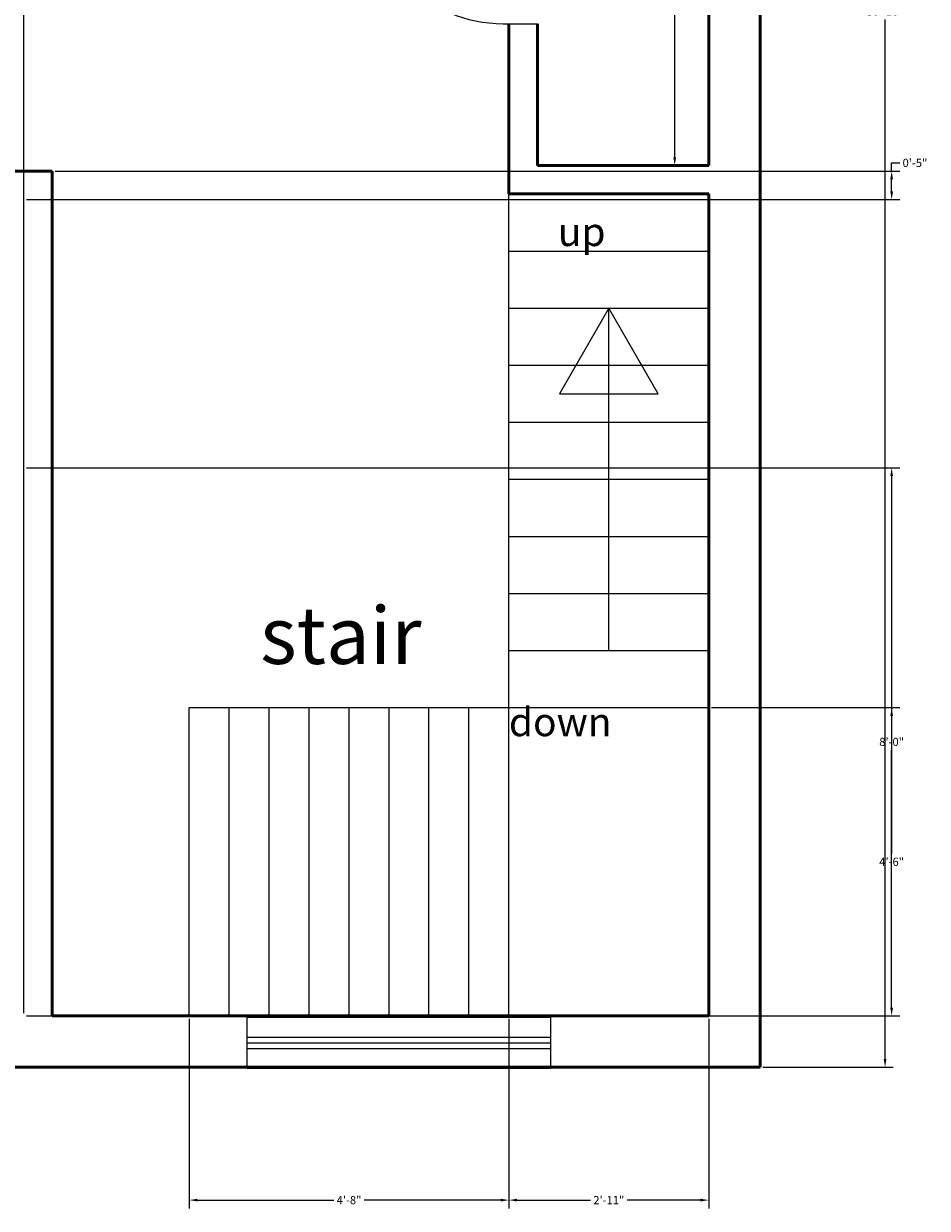
# Model space of a CAD drawing. Units: inches. Extents: x 325 to 804, y 366 to 834.
# Tile 4 of 6: x 645 to 804, y 367 to 574. Entities that reach past the tile are written whole.
import ezdxf

# ---------------------------------------------------------------- set-up
doc = ezdxf.new("R2010")
doc.units = ezdxf.units.IN
doc.header["$MEASUREMENT"] = 0
doc.layers.get('0').update_dxf_attribs({"color": 4})
for name, color, linetype, lineweight in [('A-ANNO-DIMS', 2, 'Continuous', 18), ('A-ANNO-SYMB', 2, 'Continuous', 18), ('A-ANNO-TEXT', 7, 'Continuous', 18), ('A-AREA-IDEN', 7, 'Continuous', 25), ('A-FLOR-STRS', 4, 'Continuous', 25), ('A-WALL', 7, 'Continuous', 50), ('door', 10, 'Continuous', 25), ('window', 3, 'Continuous', 18)]:
    doc.layers.add(name, color=color, linetype=linetype, lineweight=lineweight)
doc.styles.get("Standard").update_dxf_attribs({"font": 'arial.ttf'})
doc.dimstyles.get("Standard").update_dxf_attribs({"dimscale": 8, "dimtxt": 0.18, "dimasz": 0.18, "dimexe": 0.18, "dimexo": 0.0625, "dimgap": 0.09, "dimtad": 0, "dimtih": 1, "dimtoh": 1, "dimdec": 0, "dimzin": 0, "dimdsep": 46, "dimlunit": 3, "dimtxsty": 'Standard', "dimcen": 0.09, "dimadec": 0, "dimazin": 0, "dimtfac": 1, "dimtdec": 0, "dimtofl": 0, "dimtmove": 0, "dimatfit": 3, "dimfxl": 1, "dimtolj": 1, "dimtzin": 0, "dimarcsym": 0})

# ---------------------------------------------------------------- blocks, each defined once
blk = doc.blocks.new('*U8')
for p, q in [((-24, 0), (-24, -6)), ((0, 0), (0, -6))]:
    blk.add_line(p, q)
blk.add_lwpolyline([(0, 0), (0, 24), (-1.75, 24), (-1.75, 0)], close=True)
blk.add_arc((0, 0), 24, 90, 180)
blk = doc.blocks.new('*D21')
at = {"layer": 'A-ANNO-DIMS', "color": 0, "lineweight": -2, "transparency": 16777216}
for p, q in [((764.97, 609.54), (758.08, 609.54)), ((759.52, 608.1), (759.52, 580.99)), ((759.52, 550.98), (759.52, 578.09)), ((764.97, 549.54), (758.08, 549.54))]:
    blk.add_line(p, q, dxfattribs=at)
at = {"layer": 'A-ANNO-DIMS', "color": 0, "transparency": 16777216}
for points in [[(759.28, 608.1), (759.76, 608.1), (759.52, 609.54)], [(759.28, 550.98), (759.76, 550.98), (759.52, 549.54)]]:
    blk.add_solid(points, dxfattribs=at)
at = {"layer": 'Defpoints', "color": 0, "transparency": 16777216}
for p in [(765.47, 609.54), (759.52, 549.54), (765.47, 549.54)]:
    blk.add_point(p, dxfattribs=at)
at = {"layer": 'A-ANNO-DIMS', "color": 0, "transparency": 16777216, "insert": (759.52, 579.54), "char_height": 1.44, "attachment_point": 5}
blk.add_mtext("\\A1;5'", dxfattribs=at)
blk = doc.blocks.new('*D26')
at = {"layer": 'A-ANNO-DIMS', "color": 0, "lineweight": -2, "transparency": 16777216}
for p, q in [((774.97, 761.54), (797.81, 761.54)), ((796.37, 760.1), (796.37, 577.99)), ((796.37, 392.98), (796.37, 575.08)), ((774.97, 391.54), (797.81, 391.54))]:
    blk.add_line(p, q, dxfattribs=at)
at = {"layer": 'A-ANNO-DIMS', "color": 0, "transparency": 16777216}
for points in [[(796.13, 760.1), (796.61, 760.1), (796.37, 761.54)], [(796.13, 392.98), (796.61, 392.98), (796.37, 391.54)]]:
    blk.add_solid(points, dxfattribs=at)
at = {"layer": 'Defpoints', "color": 0, "transparency": 16777216}
for p in [(774.47, 761.54), (774.47, 391.54), (796.37, 391.54)]:
    blk.add_point(p, dxfattribs=at)
at = {"layer": 'A-ANNO-DIMS', "color": 0, "transparency": 16777216, "insert": (796.37, 576.54), "char_height": 1.44, "attachment_point": 5}
blk.add_mtext('\\A1;30\'-10"', dxfattribs=at)
blk = doc.blocks.new('WIN-53_14x9')
for p, q in [((0, 5.5), (53.14, 5.5)), ((0, 4.5), (53.14, 4.5)), ((0, 3.5), (53.14, 3.5))]:
    blk.add_line(p, q)
blk.add_lwpolyline([(0, 9), (53.14, 9), (53.14, 0), (0, 0)], close=True)
blk = doc.blocks.new('*D38')
at = {"layer": 'A-ANNO-DIMS', "color": 0, "lineweight": -2, "transparency": 16777216}
for p, q in [((585.47, 401.04), (585.47, 786.03)), ((586.91, 784.59), (612.84, 784.59)), ((644.03, 784.59), (618.11, 784.59)), ((645.47, 401.04), (645.47, 786.03))]:
    blk.add_line(p, q, dxfattribs=at)
at = {"layer": 'A-ANNO-DIMS', "color": 0, "transparency": 16777216}
for points in [[(586.91, 784.83), (586.91, 784.35), (585.47, 784.59)], [(644.03, 784.83), (644.03, 784.35), (645.47, 784.59)]]:
    blk.add_solid(points, dxfattribs=at)
at = {"layer": 'Defpoints', "color": 0, "transparency": 16777216}
for p in [(645.47, 784.59), (585.47, 400.54), (645.47, 400.54)]:
    blk.add_point(p, dxfattribs=at)
at = {"layer": 'A-ANNO-DIMS', "color": 0, "transparency": 16777216, "insert": (615.47, 784.59), "char_height": 1.44, "attachment_point": 5}
blk.add_mtext('\\A1;5\'-0"', dxfattribs=at)
blk = doc.blocks.new('*D39')
at = {"layer": 'A-ANNO-DIMS', "color": 0, "lineweight": -2, "transparency": 16777216}
for p, q in [((645.97, 496.54), (798.96, 496.54)), ((797.52, 495.1), (797.52, 449.99)), ((797.52, 401.98), (797.52, 447.08)), ((645.97, 400.54), (798.96, 400.54))]:
    blk.add_line(p, q, dxfattribs=at)
at = {"layer": 'A-ANNO-DIMS', "color": 0, "transparency": 16777216}
for points in [[(797.28, 495.1), (797.76, 495.1), (797.52, 496.54)], [(797.28, 401.98), (797.76, 401.98), (797.52, 400.54)]]:
    blk.add_solid(points, dxfattribs=at)
at = {"layer": 'Defpoints', "color": 0, "transparency": 16777216}
for p in [(645.47, 496.54), (797.52, 496.54), (645.47, 400.54)]:
    blk.add_point(p, dxfattribs=at)
at = {"layer": 'A-ANNO-DIMS', "color": 0, "transparency": 16777216, "insert": (797.52, 448.54), "char_height": 1.44, "attachment_point": 5}
blk.add_mtext('\\A1;8\'-0"', dxfattribs=at)
blk = doc.blocks.new('*D42')
at = {"layer": 'A-ANNO-DIMS', "color": 0, "lineweight": -2, "transparency": 16777216}
for p, q in [((730.47, 400.04), (730.47, 366.82)), ((765.47, 400.04), (765.47, 366.82)), ((731.91, 368.26), (744.77, 368.26)), ((764.03, 368.26), (751.18, 368.26))]:
    blk.add_line(p, q, dxfattribs=at)
at = {"layer": 'A-ANNO-DIMS', "color": 0, "transparency": 16777216}
for points in [[(731.91, 368.5), (731.91, 368.02), (730.47, 368.26)], [(764.03, 368.5), (764.03, 368.02), (765.47, 368.26)]]:
    blk.add_solid(points, dxfattribs=at)
at = {"layer": 'Defpoints', "color": 0, "transparency": 16777216}
for p in [(730.47, 400.54), (765.47, 400.54), (765.47, 368.26)]:
    blk.add_point(p, dxfattribs=at)
at = {"layer": 'A-ANNO-DIMS', "color": 0, "transparency": 16777216, "insert": (747.97, 368.26), "char_height": 1.44, "attachment_point": 5}
blk.add_mtext('\\A1;2\'-11"', dxfattribs=at)
blk = doc.blocks.new('*D43')
at = {"layer": 'A-ANNO-DIMS', "color": 0, "lineweight": -2, "transparency": 16777216}
for p, q in [((674.47, 400.04), (674.47, 366.82)), ((730.47, 400.04), (730.47, 366.82)), ((675.91, 368.26), (699.81, 368.26)), ((729.03, 368.26), (705.14, 368.26))]:
    blk.add_line(p, q, dxfattribs=at)
at = {"layer": 'A-ANNO-DIMS', "color": 0, "transparency": 16777216}
for points in [[(675.91, 368.5), (675.91, 368.02), (674.47, 368.26)], [(729.03, 368.5), (729.03, 368.02), (730.47, 368.26)]]:
    blk.add_solid(points, dxfattribs=at)
at = {"layer": 'Defpoints', "color": 0, "transparency": 16777216}
for p in [(674.47, 400.54), (730.47, 400.54), (730.47, 368.26)]:
    blk.add_point(p, dxfattribs=at)
at = {"layer": 'A-ANNO-DIMS', "color": 0, "transparency": 16777216, "insert": (702.47, 368.26), "char_height": 1.44, "attachment_point": 5}
blk.add_mtext('\\A1;4\'-8"', dxfattribs=at)
blk = doc.blocks.new('*D44')
at = {"layer": 'A-ANNO-DIMS', "color": 0, "lineweight": -2, "transparency": 16777216}
for p, q in [((765.97, 454.54), (798.96, 454.54)), ((797.52, 453.1), (797.52, 428.99)), ((797.52, 401.98), (797.52, 426.08)), ((765.97, 400.54), (798.96, 400.54))]:
    blk.add_line(p, q, dxfattribs=at)
at = {"layer": 'A-ANNO-DIMS', "color": 0, "transparency": 16777216}
for points in [[(797.28, 453.1), (797.76, 453.1), (797.52, 454.54)], [(797.28, 401.98), (797.76, 401.98), (797.52, 400.54)]]:
    blk.add_solid(points, dxfattribs=at)
at = {"layer": 'Defpoints', "color": 0, "transparency": 16777216}
for p in [(765.47, 454.54), (765.47, 400.54), (797.52, 400.54)]:
    blk.add_point(p, dxfattribs=at)
at = {"layer": 'A-ANNO-DIMS', "color": 0, "transparency": 16777216, "insert": (797.52, 427.54), "char_height": 1.44, "attachment_point": 5}
blk.add_mtext('\\A1;4\'-6"', dxfattribs=at)
blk = doc.blocks.new('*D47')
at = {"layer": 'A-ANNO-DIMS', "color": 0, "lineweight": -2, "transparency": 16777216}
for p, q in [((650.97, 548.54), (798.96, 548.54)), ((797.52, 548.54), (797.52, 549.98)), ((797.52, 549.98), (798.96, 549.98)), ((797.52, 544.98), (797.52, 547.1)), ((645.97, 543.54), (798.96, 543.54))]:
    blk.add_line(p, q, dxfattribs=at)
at = {"layer": 'A-ANNO-DIMS', "color": 0, "transparency": 16777216}
for points in [[(797.28, 547.1), (797.76, 547.1), (797.52, 548.54)], [(797.28, 544.98), (797.76, 544.98), (797.52, 543.54)]]:
    blk.add_solid(points, dxfattribs=at)
at = {"layer": 'Defpoints', "color": 0, "transparency": 16777216}
for p in [(650.47, 548.54), (797.52, 548.54), (645.47, 543.54)]:
    blk.add_point(p, dxfattribs=at)
at = {"layer": 'A-ANNO-DIMS', "color": 0, "transparency": 16777216, "insert": (801.6, 549.98), "char_height": 1.44, "attachment_point": 5}
blk.add_mtext('\\A1;0\'-5"', dxfattribs=at)

msp = doc.modelspace()

# ---------------------------------------------------------------- linework, layer by layer
at = {"layer": 'A-ANNO-SYMB'}
msp.add_line((747.97, 464.54), (747.97, 524.54), dxfattribs=at)
msp.add_lwpolyline([(747.97, 524.54), (739.31, 509.54), (756.63, 509.54)], close=True, dxfattribs=at)
at = {"layer": 'A-FLOR-STRS'}
for p, q in [((730.47, 400.54), (730.47, 544.54)), ((730.47, 534.54), (765.47, 534.54)), ((730.47, 524.54), (765.47, 524.54)), ((730.47, 514.54), (765.47, 514.54)), ((730.47, 504.54), (765.47, 504.54)), ((730.47, 494.54), (765.47, 494.54)), ((730.47, 484.54), (765.47, 484.54)), ((730.47, 474.54), (765.47, 474.54)), ((730.47, 464.54), (765.47, 464.54)), ((674.47, 454.54), (765.47, 454.54)), ((674.47, 400.54), (674.47, 454.54)), ((681.47, 400.54), (681.47, 454.54)), ((688.47, 400.54), (688.47, 454.54)), ((695.47, 400.54), (695.47, 454.54)), ((702.47, 400.54), (702.47, 454.54)), ((709.47, 400.54), (709.47, 454.54)), ((716.47, 400.54), (716.47, 454.54)), ((723.47, 400.54), (723.47, 454.54))]:
    msp.add_line(p, q, dxfattribs=at)
at = {"layer": 'A-WALL'}
for p, q in [((774.47, 391.54), (774.47, 761.54)), ((765.47, 549.54), (765.47, 609.54)), ((730.47, 574.37), (730.47, 544.54)), ((735.47, 574.37), (735.47, 549.54)), ((538.47, 548.54), (650.47, 548.54)), ((650.47, 400.54), (650.47, 548.54)), ((735.47, 549.54), (765.47, 549.54)), ((730.47, 544.54), (765.47, 544.54)), ((765.47, 453.67), (765.47, 544.54)), ((765.47, 400.54), (765.47, 453.67)), ((650.47, 400.54), (765.47, 400.54)), ((350.47, 391.54), (774.47, 391.54))]:
    msp.add_line(p, q, dxfattribs=at)

# ---------------------------------------------------------------- block references
at = {"layer": 'door', "rotation": 90}
msp.add_blockref('*U8', (729.47, 598.37), dxfattribs=at)
at = {"layer": 'window'}
msp.add_blockref('WIN-53_14x9', (684.61, 391.31), dxfattribs=at)

# ---------------------------------------------------------------- texts
at = {"layer": 'A-ANNO-TEXT', "char_height": 5, "attachment_point": 1}
for s, width, insert in [('up', 26.4321, (739.04, 540.41)), ('down', 35, (730.47, 454.54))]:
    msp.add_mtext_dynamic_manual_height_columns(s, width=width, gutter_width=1, heights=[0], dxfattribs=dict(at, insert=insert))
at = {"layer": 'A-AREA-IDEN', "insert": (686.9, 472.2), "char_height": 10, "attachment_point": 1}
msp.add_mtext_dynamic_manual_height_columns('stair', width=14.76, gutter_width=1, heights=[0], dxfattribs=at)

# ---------------------------------------------------------------- dimensions: what is measured, and where the dimension line sits
at = {"layer": 'A-ANNO-DIMS'}
for base, p1, p2, picture, middle in [((645.47, 784.59), (585.47, 400.54), (645.47, 400.54), '*D38', (615.47, 784.59)), ((730.47, 368.26), (674.47, 400.54), (730.47, 400.54), '*D43', (702.47, 368.26)), ((765.47, 368.26), (730.47, 400.54), (765.47, 400.54), '*D42', (747.97, 368.26))]:
    dim = msp.add_linear_dim(base=base, p1=p1, p2=p2, dimstyle='Standard', override={"dimdec": 1, "dimlfac": 1, "dimrnd": 0, "dimzin": 1, "dimdsep": 46, "dimlunit": 4, "dimfrac": 2}, dxfattribs=at)
    dim.commit()
    dim.dimension.update_dxf_attribs({"geometry": picture, "text_midpoint": middle})
for base, p1, p2, override, picture, middle in [((796.37, 391.54), (774.47, 761.54), (774.47, 391.54), {"dimclrd": 0, "dimclre": 0, "dimclrt": 0}, '*D26', (796.37, 576.54)), ((759.52, 549.54), (765.47, 609.54), (765.47, 549.54), {"dimclrd": 0, "dimclre": 0, "dimclrt": 0}, '*D21', (759.52, 579.54)), ((797.52, 548.54), (645.47, 543.54), (650.47, 548.54), {"dimdec": 1, "dimlfac": 1, "dimrnd": 0, "dimzin": 1, "dimdsep": 46, "dimlunit": 4, "dimfrac": 2}, '*D47', (801.6, 549.98)), ((797.52, 496.54), (645.47, 400.54), (645.47, 496.54), {"dimdec": 1, "dimlfac": 1, "dimrnd": 0, "dimzin": 1, "dimdsep": 46, "dimlunit": 4, "dimfrac": 2}, '*D39', (797.52, 448.54)), ((797.52, 400.54), (765.47, 454.54), (765.47, 400.54), {"dimdec": 1, "dimlfac": 1, "dimrnd": 0, "dimzin": 1, "dimdsep": 46, "dimlunit": 4, "dimfrac": 2}, '*D44', (797.52, 427.54))]:
    dim = msp.add_linear_dim(base=base, p1=p1, p2=p2, angle=90, dimstyle='Standard', override=override, dxfattribs=at)
    dim.commit()
    dim.dimension.update_dxf_attribs({"geometry": picture, "text_midpoint": middle})

doc.saveas('drawing.dxf')
